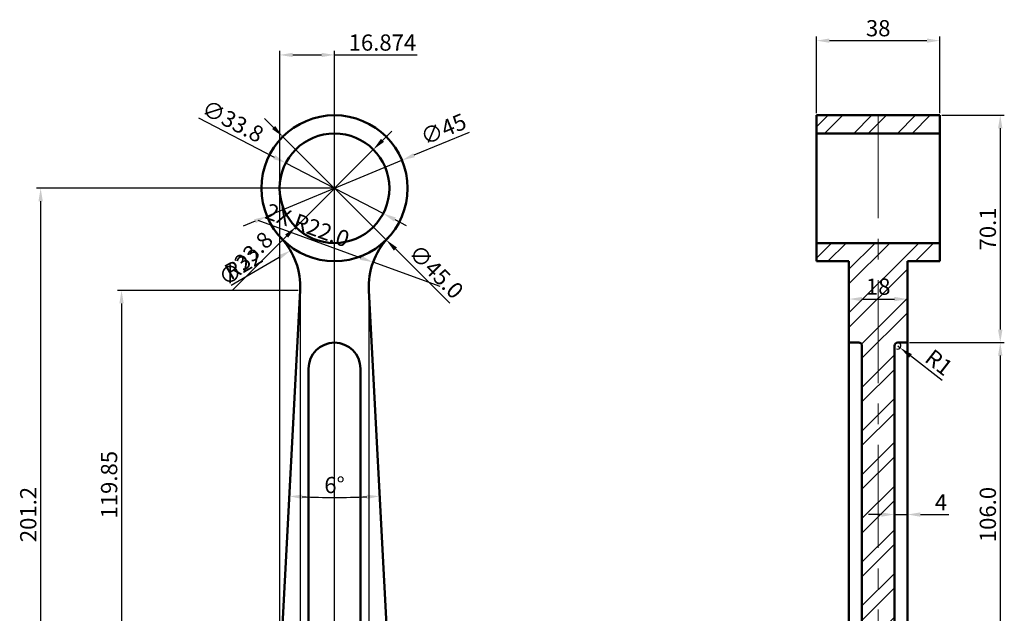
# Model space of a CAD drawing. Units: millimetres. Extents: x 3127 to 3430, y 1464 to 1830.
# Tile 2 of 2: x 3127 to 3430, y 1647 to 1830. Entities that reach past the tile are written whole.
import ezdxf

# ---------------------------------------------------------------- set-up
doc = ezdxf.new("R2010")
doc.units = ezdxf.units.MM
doc.linetypes.add('CENTER', pattern=[50.8, 31.75, -6.35, 6.35, -6.35])
for name, color, linetype, lineweight in [('M-CNTR', 1, 'CENTER', 18), ('M-DIMS', 2, 'Continuous', 25), ('M-HATC', 8, 'Continuous', 18), ('M-OUTL', 7, 'Continuous', 50)]:
    doc.layers.add(name, color=color, linetype=linetype, lineweight=lineweight)
doc.styles.get("Standard").update_dxf_attribs({"font": 'arial.ttf'})
doc.dimstyles.new('ISO-25', dxfattribs={"dimtxt": 5, "dimasz": 4, "dimexe": 1.25, "dimexo": 0.625, "dimtad": 1, "dimdsep": 46, "dimtxsty": 'Standard', "dimcen": 2.5, "dimadec": 0, "dimazin": 0, "dimtfac": 1, "dimtmove": 0, "dimatfit": 3, "dimfxl": 1, "dimarcsym": 0})

# ---------------------------------------------------------------- blocks, each defined once
blk = doc.blocks.new('*D3')
at = {"layer": 'Defpoints', "color": 0, "transparency": 16777216}
for p in [(3396.63, 1677.1), (3400.63, 1677.1), (3400.63, 1677.1)]:
    blk.add_point(p, dxfattribs=at)
at = {"layer": 'M-DIMS', "color": 0, "lineweight": -2, "transparency": 16777216}
for p, q in [((3396.63, 1677.72), (3396.63, 1678.35)), ((3400.63, 1677.72), (3400.63, 1678.35)), ((3392.63, 1677.1), (3388.63, 1677.1)), ((3396.63, 1677.1), (3400.63, 1677.1)), ((3404.63, 1677.1), (3413.34, 1677.1))]:
    blk.add_line(p, q, dxfattribs=at)
at = {"layer": 'M-DIMS', "color": 0, "transparency": 16777216}
for points in [[(3392.63, 1677.76), (3392.63, 1676.43), (3396.63, 1677.1)], [(3404.63, 1677.76), (3404.63, 1676.43), (3400.63, 1677.1)]]:
    blk.add_solid(points, dxfattribs=at)
at = {"layer": 'M-DIMS', "color": 0, "transparency": 16777216, "insert": (3410.98, 1680.22), "char_height": 5, "attachment_point": 5}
blk.add_mtext('4', dxfattribs=at)
blk = doc.blocks.new('*D12')
at = {"layer": 'Defpoints', "color": 0, "transparency": 16777216}
for p in [(3213.56, 1746.21), (3234.74, 1746.21), (3219.51, 1682.41), (3207.27, 1626.37), (3241.02, 1626.37)]:
    blk.add_point(p, dxfattribs=at)
at = {"layer": 'M-DIMS', "color": 0, "lineweight": -2, "transparency": 16777216}
blk.add_arc((3224.15, 1948.35), 265.98, 267.8617, 272.1383, dxfattribs=at)
at = {"layer": 'M-DIMS', "color": 0, "transparency": 16777216}
for points in [[(3214.19, 1681.89), (3214.25, 1683.22), (3210.23, 1682.73)], [(3234.04, 1683.22), (3234.1, 1681.89), (3238.07, 1682.73)]]:
    blk.add_solid(points, dxfattribs=at)
at = {"layer": 'M-DIMS', "color": 0, "transparency": 16777216, "insert": (3224.15, 1685.55), "char_height": 5, "attachment_point": 5}
blk.add_mtext('6°', dxfattribs=at)
blk = doc.blocks.new('*D13')
at = {"layer": 'Defpoints', "color": 0, "transparency": 16777216}
for p in [(3210.59, 1758.45), (3191.59, 1747.37)]:
    blk.add_point(p, dxfattribs=at)
at = {"layer": 'M-DIMS', "color": 0, "lineweight": -2, "transparency": 16777216}
blk.add_line((3192.32, 1747.8), (3207.13, 1756.43), dxfattribs=at)
at = {"layer": 'M-DIMS', "color": 0, "transparency": 16777216}
blk.add_solid([(3206.8, 1757.01), (3207.47, 1755.86), (3210.59, 1758.45)], dxfattribs=at)
at = {"layer": 'M-DIMS', "color": 0, "transparency": 16777216, "insert": (3196.42, 1753.82), "char_height": 5, "attachment_point": 5, "rotation": 30.2469}
blk.add_mtext('R22', dxfattribs=at)
blk = doc.blocks.new('*D14')
at = {"layer": 'Defpoints', "color": 0, "transparency": 16777216}
for p in [(3244.93, 1786.33), (3203.37, 1769.06)]:
    blk.add_point(p, dxfattribs=at)
at = {"layer": 'M-DIMS', "color": 0, "lineweight": -2, "transparency": 16777216}
for p, q in [((3265.64, 1794.93), (3248.62, 1787.86)), ((3203.37, 1769.06), (3244.93, 1786.33)), ((3199.68, 1767.53), (3195.98, 1766))]:
    blk.add_line(p, q, dxfattribs=at)
at = {"layer": 'M-DIMS', "color": 0, "transparency": 16777216}
for points in [[(3248.37, 1788.48), (3248.88, 1787.25), (3244.93, 1786.33)], [(3199.42, 1768.15), (3199.93, 1766.91), (3203.37, 1769.06)]]:
    blk.add_solid(points, dxfattribs=at)
at = {"layer": 'M-DIMS', "color": 0, "transparency": 16777216, "insert": (3257.95, 1795.33), "char_height": 5, "attachment_point": 5, "rotation": 22.5579}
blk.add_mtext('∅45', dxfattribs=at)
blk = doc.blocks.new('*D15')
at = {"layer": 'Defpoints', "color": 0, "transparency": 16777216}
for p in [(3209.14, 1785.47), (3239.16, 1769.92)]:
    blk.add_point(p, dxfattribs=at)
at = {"layer": 'M-DIMS', "color": 0, "lineweight": -2, "transparency": 16777216}
for p, q in [((3182.26, 1799.39), (3205.59, 1787.31)), ((3239.16, 1769.92), (3209.14, 1785.47)), ((3242.71, 1768.09), (3246.26, 1766.25))]:
    blk.add_line(p, q, dxfattribs=at)
at = {"layer": 'M-DIMS', "color": 0, "transparency": 16777216}
for points in [[(3205.9, 1787.9), (3205.28, 1786.71), (3209.14, 1785.47)], [(3243.01, 1768.68), (3242.4, 1767.49), (3239.16, 1769.92)]]:
    blk.add_solid(points, dxfattribs=at)
at = {"layer": 'M-DIMS', "color": 0, "transparency": 16777216, "insert": (3192.53, 1797.81), "char_height": 5, "attachment_point": 5, "rotation": 332.6249}
blk.add_mtext('∅33.8', dxfattribs=at)
blk = doc.blocks.new('*D16')
at = {"layer": 'Defpoints', "color": 0, "transparency": 16777216}
for p in [(3224.15, 1777.7), (3133.63, 1576.5), (3177.15, 1576.5)]:
    blk.add_point(p, dxfattribs=at)
at = {"layer": 'M-DIMS', "color": 0, "lineweight": -2, "transparency": 16777216}
for p, q in [((3223.52, 1777.7), (3132.38, 1777.7)), ((3133.63, 1773.7), (3133.63, 1580.5)), ((3176.52, 1576.5), (3132.38, 1576.5))]:
    blk.add_line(p, q, dxfattribs=at)
at = {"layer": 'M-DIMS', "color": 0, "transparency": 16777216}
for points in [[(3132.96, 1773.7), (3134.3, 1773.7), (3133.63, 1777.7)], [(3132.96, 1580.5), (3134.3, 1580.5), (3133.63, 1576.5)]]:
    blk.add_solid(points, dxfattribs=at)
at = {"layer": 'M-DIMS', "color": 0, "transparency": 16777216, "insert": (3130.45, 1677.1), "char_height": 5, "attachment_point": 5, "rotation": 90}
blk.add_mtext('201.2', dxfattribs=at)
blk = doc.blocks.new('*D17')
at = {"layer": 'Defpoints', "color": 0, "transparency": 16777216}
for p in [(3382.63, 1743.53), (3400.63, 1743.53), (3400.63, 1743.53)]:
    blk.add_point(p, dxfattribs=at)
at = {"layer": 'M-DIMS', "color": 0, "lineweight": -2, "transparency": 16777216}
for p, q in [((3382.63, 1744.15), (3382.63, 1744.78)), ((3400.63, 1744.15), (3400.63, 1744.78)), ((3386.63, 1743.53), (3396.63, 1743.53))]:
    blk.add_line(p, q, dxfattribs=at)
at = {"layer": 'M-DIMS', "color": 0, "transparency": 16777216}
for points in [[(3386.63, 1744.2), (3386.63, 1742.86), (3382.63, 1743.53)], [(3396.63, 1744.2), (3396.63, 1742.86), (3400.63, 1743.53)]]:
    blk.add_solid(points, dxfattribs=at)
at = {"layer": 'M-DIMS', "color": 0, "transparency": 16777216, "insert": (3391.63, 1746.71), "char_height": 5, "attachment_point": 5}
blk.add_mtext('18', dxfattribs=at)
blk = doc.blocks.new('*D18')
at = {"layer": 'Defpoints', "color": 0, "transparency": 16777216}
for p in [(3397.63, 1729.1), (3398.42, 1728.48)]:
    blk.add_point(p, dxfattribs=at)
at = {"layer": 'M-DIMS', "color": 0, "lineweight": -2, "transparency": 16777216}
for p, q in [((3397.63, 1729.1), (3398.42, 1728.48)), ((3411.32, 1718.44), (3401.58, 1726.03))]:
    blk.add_line(p, q, dxfattribs=at)
blk.add_arc((3397.63, 1729.1), 1, 250.5029, 54.1901, dxfattribs=at)
at = {"layer": 'M-DIMS', "color": 0, "transparency": 16777216}
blk.add_solid([(3401.99, 1726.55), (3401.17, 1725.5), (3398.42, 1728.48)], dxfattribs=at)
at = {"layer": 'M-DIMS', "color": 0, "transparency": 16777216, "insert": (3409.95, 1723.48), "char_height": 5, "attachment_point": 5, "rotation": 322.1226}
blk.add_mtext('R1', dxfattribs=at)
blk = doc.blocks.new('*D19')
at = {"layer": 'Defpoints', "color": 0, "transparency": 16777216}
for p in [(3410.63, 1823.21), (3372.63, 1800.2), (3410.63, 1800.2)]:
    blk.add_point(p, dxfattribs=at)
at = {"layer": 'M-DIMS', "color": 0, "lineweight": -2, "transparency": 16777216}
for p, q in [((3372.63, 1800.82), (3372.63, 1824.46)), ((3376.63, 1823.21), (3406.63, 1823.21)), ((3410.63, 1800.82), (3410.63, 1824.46))]:
    blk.add_line(p, q, dxfattribs=at)
at = {"layer": 'M-DIMS', "color": 0, "transparency": 16777216}
for points in [[(3376.63, 1823.88), (3376.63, 1822.54), (3372.63, 1823.21)], [(3406.63, 1823.88), (3406.63, 1822.54), (3410.63, 1823.21)]]:
    blk.add_solid(points, dxfattribs=at)
at = {"layer": 'M-DIMS', "color": 0, "transparency": 16777216, "insert": (3391.63, 1826.39), "char_height": 5, "attachment_point": 5}
blk.add_mtext('38', dxfattribs=at)
blk = doc.blocks.new('*D22')
at = {"layer": 'Defpoints', "color": 0, "transparency": 16777216}
for p in [(3410.63, 1800.2), (3400.63, 1730.1), (3429.23, 1730.1)]:
    blk.add_point(p, dxfattribs=at)
at = {"layer": 'M-DIMS', "color": 0, "lineweight": -2, "transparency": 16777216}
for p, q in [((3411.25, 1800.2), (3430.48, 1800.2)), ((3429.23, 1796.2), (3429.23, 1734.1)), ((3401.25, 1730.1), (3430.48, 1730.1))]:
    blk.add_line(p, q, dxfattribs=at)
at = {"layer": 'M-DIMS', "color": 0, "transparency": 16777216}
for points in [[(3428.56, 1796.2), (3429.9, 1796.2), (3429.23, 1800.2)], [(3428.56, 1734.1), (3429.9, 1734.1), (3429.23, 1730.1)]]:
    blk.add_solid(points, dxfattribs=at)
at = {"layer": 'M-DIMS', "color": 0, "transparency": 16777216, "insert": (3426.05, 1765.15), "char_height": 5, "attachment_point": 5, "rotation": 90}
blk.add_mtext('70.1', dxfattribs=at)
blk = doc.blocks.new('*D23')
at = {"layer": 'Defpoints', "color": 0, "transparency": 16777216}
for p in [(3400.63, 1730.1), (3400.63, 1624.1), (3429.23, 1624.1)]:
    blk.add_point(p, dxfattribs=at)
at = {"layer": 'M-DIMS', "color": 0, "lineweight": -2, "transparency": 16777216}
for p, q in [((3401.25, 1730.1), (3430.48, 1730.1)), ((3429.23, 1726.1), (3429.23, 1628.1)), ((3401.25, 1624.1), (3430.48, 1624.1))]:
    blk.add_line(p, q, dxfattribs=at)
at = {"layer": 'M-DIMS', "color": 0, "transparency": 16777216}
for points in [[(3428.56, 1726.1), (3429.9, 1726.1), (3429.23, 1730.1)], [(3428.56, 1628.1), (3429.9, 1628.1), (3429.23, 1624.1)]]:
    blk.add_solid(points, dxfattribs=at)
at = {"layer": 'M-DIMS', "color": 0, "transparency": 16777216, "insert": (3426.05, 1677.1), "char_height": 5, "attachment_point": 5, "rotation": 90}
blk.add_mtext('106.0', dxfattribs=at)
blk = doc.blocks.new('*D24')
at = {"layer": 'Defpoints', "color": 0, "transparency": 16777216}
for p in [(3213.56, 1746.21), (3234.74, 1746.21), (3234.74, 1469.62)]:
    blk.add_point(p, dxfattribs=at)
at = {"layer": 'M-DIMS', "color": 0, "lineweight": -2, "transparency": 16777216}
for p, q in [((3213.56, 1745.59), (3213.56, 1468.37)), ((3234.74, 1745.59), (3234.74, 1468.37)), ((3217.56, 1469.62), (3230.74, 1469.62)), ((3234.74, 1469.62), (3260.83, 1469.62))]:
    blk.add_line(p, q, dxfattribs=at)
at = {"layer": 'M-DIMS', "color": 0, "transparency": 16777216}
for points in [[(3217.56, 1470.29), (3217.56, 1468.96), (3213.56, 1469.62)], [(3230.74, 1470.29), (3230.74, 1468.96), (3234.74, 1469.62)]]:
    blk.add_solid(points, dxfattribs=at)
at = {"layer": 'M-DIMS', "color": 0, "transparency": 16777216, "insert": (3249.79, 1472.8), "char_height": 5, "attachment_point": 5}
blk.add_mtext('21.187', dxfattribs=at)
blk = doc.blocks.new('*D25')
at = {"layer": 'Defpoints', "color": 0, "transparency": 16777216}
for p in [(3224.15, 1818.8), (3207.27, 1626.37), (3224.15, 1603.5)]:
    blk.add_point(p, dxfattribs=at)
at = {"layer": 'M-DIMS', "color": 0, "lineweight": -2, "transparency": 16777216}
for p, q in [((3207.27, 1626.99), (3207.27, 1820.05)), ((3224.15, 1604.12), (3224.15, 1820.05)), ((3211.27, 1818.8), (3220.15, 1818.8)), ((3224.15, 1818.8), (3249.66, 1818.8))]:
    blk.add_line(p, q, dxfattribs=at)
at = {"layer": 'M-DIMS', "color": 0, "transparency": 16777216}
for points in [[(3211.27, 1819.46), (3211.27, 1818.13), (3207.27, 1818.8)], [(3220.15, 1819.46), (3220.15, 1818.13), (3224.15, 1818.8)]]:
    blk.add_solid(points, dxfattribs=at)
at = {"layer": 'M-DIMS', "color": 0, "transparency": 16777216, "insert": (3238.91, 1821.97), "char_height": 5, "attachment_point": 5}
blk.add_mtext('16.874', dxfattribs=at)
blk = doc.blocks.new('*D26')
at = {"layer": 'Defpoints', "color": 0, "transparency": 16777216}
for p in [(3213.56, 1746.21), (3158.55, 1626.37), (3207.27, 1626.37)]:
    blk.add_point(p, dxfattribs=at)
at = {"layer": 'M-DIMS', "color": 0, "lineweight": -2, "transparency": 16777216}
for p, q in [((3212.93, 1746.21), (3157.3, 1746.21)), ((3158.55, 1742.21), (3158.55, 1630.37)), ((3206.65, 1626.37), (3157.3, 1626.37))]:
    blk.add_line(p, q, dxfattribs=at)
at = {"layer": 'M-DIMS', "color": 0, "transparency": 16777216}
for points in [[(3157.88, 1742.21), (3159.22, 1742.21), (3158.55, 1746.21)], [(3157.88, 1630.37), (3159.22, 1630.37), (3158.55, 1626.37)]]:
    blk.add_solid(points, dxfattribs=at)
at = {"layer": 'M-DIMS', "color": 0, "transparency": 16777216, "insert": (3155.37, 1686.29), "char_height": 5, "attachment_point": 5, "rotation": 90}
blk.add_mtext('119.85', dxfattribs=at)
blk = doc.blocks.new('*D28')
at = {"layer": 'Defpoints', "color": 0, "transparency": 16777216}
for p in [(3208.23, 1793.6), (3240.07, 1761.79)]:
    blk.add_point(p, dxfattribs=at)
at = {"layer": 'M-DIMS', "color": 0, "lineweight": -2, "transparency": 16777216}
for p, q in [((3205.4, 1796.42), (3202.57, 1799.25)), ((3208.23, 1793.6), (3240.07, 1761.79)), ((3259.64, 1742.24), (3242.9, 1758.97))]:
    blk.add_line(p, q, dxfattribs=at)
at = {"layer": 'M-DIMS', "color": 0, "transparency": 16777216}
for points in [[(3205.87, 1796.9), (3204.93, 1795.95), (3208.23, 1793.6)], [(3243.37, 1759.44), (3242.43, 1758.49), (3240.07, 1761.79)]]:
    blk.add_solid(points, dxfattribs=at)
at = {"layer": 'M-DIMS', "color": 0, "transparency": 16777216, "insert": (3255.03, 1751.54), "char_height": 5, "attachment_point": 5, "rotation": 315.0282}
blk.add_mtext('∅45.0', dxfattribs=at)
blk = doc.blocks.new('*D29')
at = {"layer": 'Defpoints', "color": 0, "transparency": 16777216}
for p in [(3236.1, 1789.64), (3212.2, 1765.75)]:
    blk.add_point(p, dxfattribs=at)
at = {"layer": 'M-DIMS', "color": 0, "lineweight": -2, "transparency": 16777216}
for p, q in [((3238.93, 1792.47), (3241.76, 1795.3)), ((3236.1, 1789.64), (3212.2, 1765.75)), ((3192.62, 1746.17), (3209.37, 1762.92))]:
    blk.add_line(p, q, dxfattribs=at)
at = {"layer": 'M-DIMS', "color": 0, "transparency": 16777216}
for points in [[(3238.46, 1792.94), (3239.4, 1792), (3236.1, 1789.64)], [(3208.9, 1763.39), (3209.84, 1762.45), (3212.2, 1765.75)]]:
    blk.add_solid(points, dxfattribs=at)
at = {"layer": 'M-DIMS', "color": 0, "transparency": 16777216, "insert": (3197.23, 1755.48), "char_height": 5, "attachment_point": 5, "rotation": 44.993}
blk.add_mtext('∅33.8', dxfattribs=at)
blk = doc.blocks.new('*D30')
at = {"layer": 'Defpoints', "color": 0, "transparency": 16777216}
for p in [(3236.04, 1754.88), (3256.71, 1747.37)]:
    blk.add_point(p, dxfattribs=at)
at = {"layer": 'M-DIMS', "color": 0, "lineweight": -2, "transparency": 16777216}
for p, q in [((3200.48, 1767.81), (3232.28, 1756.25)), ((3256.71, 1747.37), (3236.04, 1754.88))]:
    blk.add_line(p, q, dxfattribs=at)
at = {"layer": 'M-DIMS', "color": 0, "transparency": 16777216}
blk.add_solid([(3232.51, 1756.88), (3232.05, 1755.62), (3236.04, 1754.88)], dxfattribs=at)
at = {"layer": 'M-DIMS', "color": 0, "transparency": 16777216, "insert": (3215.58, 1765.7), "char_height": 5, "attachment_point": 5, "rotation": 340.0179}
blk.add_mtext('2X R22.0', dxfattribs=at)

msp = doc.modelspace()

# ---------------------------------------------------------------- hatches: boundary and pattern name
at = {"layer": 'M-HATC'}
h = msp.add_hatch(dxfattribs=at)
h.set_pattern_fill('ANSI32', color=256)
h.paths.add_polyline_path([(3391.6295, 1800.1957), (3372.6295, 1800.1957), (3372.6295, 1794.5957), (3391.6295, 1794.5957)])
h.paths.add_polyline_path([(3410.6295, 1800.1957), (3391.6295, 1800.1957), (3391.6295, 1794.5957), (3410.6295, 1794.5957)])
h.paths.add_polyline_path([(3400.6295, 1755.1957), (3410.6295, 1755.1957), (3410.6295, 1760.7957), (3391.6295, 1760.7957), (3391.6295, 1603.4957), (3410.6295, 1603.4957), (3410.6295, 1613.4957), (3403.6295, 1613.4957, -0.41421356), (3400.6295, 1616.4957), (3400.6295, 1624.0957), (3397.6295, 1624.0957, -0.41421356), (3396.6295, 1625.0957), (3396.6295, 1729.0957, -0.41421356), (3397.6295, 1730.0957), (3400.6295, 1730.0957)])
h.paths.add_polyline_path([(3391.6295, 1760.7957), (3372.6295, 1760.7957), (3372.6295, 1755.1957), (3382.6295, 1755.1957), (3382.6295, 1730.0957), (3385.6295, 1730.0957, -0.41421356), (3386.6295, 1729.0957), (3386.6295, 1625.0957, -0.41421356), (3385.6295, 1624.0957), (3382.6295, 1624.0957), (3382.6295, 1616.4957, -0.41421356), (3379.6295, 1613.4957), (3372.6295, 1613.4957), (3372.6295, 1603.4957), (3391.6295, 1603.4957)])
h.paths.add_polyline_path([(3262.1486, 1526.2219), (3251.1486, 1526.2219), (3251.1486, 1507.2219), (3257.6486, 1507.2219, -1), (3266.6486, 1507.2219), (3271.1486, 1507.2219, 0.41421356), (3262.1486, 1516.2219)])
h.paths.add_polyline_path([(3271.1486, 1507.2219), (3266.6486, 1507.2219, -1), (3257.6486, 1507.2219), (3251.1486, 1507.2219), (3251.1486, 1488.2219), (3262.1486, 1488.2219), (3262.1486, 1498.2219, 0.41421356)])
h.paths.add_polyline_path([(3197.1486, 1526.2219), (3186.1486, 1526.2219), (3186.1486, 1516.2219, 0.41421356), (3177.1486, 1507.2219), (3181.6486, 1507.2219, -1), (3190.6486, 1507.2219), (3197.1486, 1507.2219)])
h.paths.add_polyline_path([(3197.1486, 1507.2219), (3190.6486, 1507.2219, -1), (3181.6486, 1507.2219), (3177.1486, 1507.2219, 0.41421356), (3186.1486, 1498.2219), (3186.1486, 1488.2219), (3197.1486, 1488.2219)])

# ---------------------------------------------------------------- linework, layer by layer
at = {"layer": 'M-CNTR'}
for p, q in [((3391.6295, 1800.1957), (3391.6295, 1576.4957)), ((3224.1486, 1777.6957), (3224.1486, 1624.0957))]:
    msp.add_line(p, q, dxfattribs=at)
at = {"layer": 'M-OUTL'}
for p, q in [((3372.6295, 1800.1957), (3410.6295, 1800.1957)), ((3372.6295, 1800.1957), (3372.6295, 1755.1957)), ((3410.6295, 1800.1957), (3410.6295, 1755.1957)), ((3372.6295, 1794.5957), (3410.6295, 1794.5957)), ((3239.0026, 1760.7957), (3239.2865, 1760.7957)), ((3372.6295, 1760.7957), (3410.6295, 1760.7957)), ((3372.6295, 1755.1957), (3382.6295, 1755.1957)), ((3382.6295, 1755.1957), (3382.6295, 1616.4957)), ((3400.6295, 1755.1957), (3400.6295, 1616.4957)), ((3400.6295, 1755.1957), (3410.6295, 1755.1957)), ((3213.5551, 1746.2148), (3207.2742, 1626.369)), ((3234.7422, 1746.2148), (3241.023, 1626.369)), ((3382.6295, 1730.0957), (3385.6295, 1730.0957)), ((3386.6295, 1729.0957), (3386.6295, 1625.0957)), ((3396.6295, 1729.0957), (3396.6295, 1625.0957)), ((3397.6295, 1730.0957), (3400.6295, 1730.0957)), ((3216.1486, 1722.0957), (3216.1486, 1632.0957)), ((3232.1486, 1722.0957), (3232.1486, 1632.0957))]:
    msp.add_line(p, q, dxfattribs=at)
for radius in [22.5, 16.9]:
    msp.add_circle((3224.1486, 1777.6957), radius, dxfattribs=at)
for centre, radius, start, end in [((3191.5853, 1747.3662), 22, 357, 42.965744), ((3256.712, 1747.3662), 22, 137.034256, 183), ((3224.1486, 1722.0957), 8, 0, 180), ((3385.6295, 1729.0957), 1, 0, 90), ((3397.6295, 1729.0957), 1, 90, 180)]:
    msp.add_arc(centre, radius, start, end, dxfattribs=at)

# ---------------------------------------------------------------- dimensions: what is measured, and where the dimension line sits
at = {"layer": 'M-DIMS'}
for base, p1, p2, override, picture, middle in [((3410.6295, 1823.2101), (3372.6295, 1800.1957), (3410.6295, 1800.1957), {"dimclrd": 0, "dimclre": 0, "dimclrt": 0}, '*D19', (3391.6295, 1826.3896)), ((3224.1486, 1818.7957), (3207.2742, 1626.369), (3224.1486, 1603.4957), {"dimdec": 3, "dimlfac": 1, "dimrnd": 0, "dimzin": 0, "dimdsep": 46, "dimlunit": 2}, '*D25', (3238.9067, 1821.9736)), ((3400.6295, 1743.5294), (3382.6295, 1743.5294), (3400.6295, 1743.5294), {"dimclrd": 0, "dimclre": 0, "dimclrt": 0}, '*D17', (3391.6295, 1746.7073)), ((3234.7422, 1469.6219), (3213.5551, 1746.2148), (3234.7422, 1746.2148), {"dimdec": 3, "dimlfac": 1, "dimrnd": 0, "dimzin": 0, "dimdsep": 46, "dimlunit": 2}, '*D24', (3249.7884, 1472.7997)), ((3400.6295, 1677.0957), (3396.6295, 1677.0957), (3400.6295, 1677.0957), {"dimclrd": 0, "dimclre": 0, "dimclrt": 0}, '*D3', (3410.9837, 1680.2207))]:
    dim = msp.add_linear_dim(base=base, p1=p1, p2=p2, dimstyle='ISO-25', override=override, dxfattribs=at)
    dim.commit()
    dim.dimension.update_dxf_attribs({"geometry": picture, "text_midpoint": middle})
for p1, p2, override, picture, middle in [((3239.1561, 1769.9249), (3209.1412, 1785.4665), {"dimclrd": 0, "dimclre": 0, "dimclrt": 0}, '*D15', (3190.9999, 1794.8601)), ((3203.3701, 1769.0643), (3244.9272, 1786.3271), {"dimclrd": 0, "dimclre": 0, "dimclrt": 0}, '*D14', (3259.2215, 1792.2649)), ((3208.2309, 1793.5978), (3240.0664, 1761.7936), {"dimdec": 1, "dimlfac": 1, "dimrnd": 0, "dimzin": 0, "dimdsep": 46, "dimlunit": 2}, '*D28', (3252.6805, 1749.1919)), ((3236.1002, 1789.6443), (3212.1971, 1765.7471), {"dimdec": 1, "dimlfac": 1, "dimrnd": 0, "dimzin": 0, "dimdsep": 46, "dimlunit": 2}, '*D29', (3199.5779, 1753.131))]:
    dim = msp.add_diameter_dim_2p(p1=p1, p2=p2, dimstyle='ISO-25', override=override, dxfattribs=at)
    dim.commit()
    dim.dimension.update_dxf_attribs({"geometry": picture, "text_midpoint": middle, "dimtype": 163})
for base, p1, p2, override, picture, middle in [((3429.2295, 1730.0957), (3410.6295, 1800.1957), (3400.6295, 1730.0957), {"dimdec": 1, "dimlfac": 1, "dimrnd": 0, "dimzin": 0, "dimdsep": 46, "dimlunit": 2}, '*D22', (3426.0516, 1765.1457)), ((3133.6315, 1576.4957), (3224.1486, 1777.6957), (3177.1486, 1576.4957), {"dimclrd": 0, "dimclre": 0, "dimclrt": 0}, '*D16', (3130.4537, 1677.0957)), ((3158.5486, 1626.369), (3213.5551, 1746.2148), (3207.2742, 1626.369), {"dimdec": 2, "dimlfac": 1, "dimrnd": 0, "dimzin": 0, "dimdsep": 46, "dimlunit": 2}, '*D26', (3155.3708, 1686.2919)), ((3429.2295, 1624.0957), (3400.6295, 1730.0957), (3400.6295, 1624.0957), {"dimdec": 1, "dimlfac": 1, "dimrnd": 0, "dimzin": 0, "dimdsep": 46, "dimlunit": 2}, '*D23', (3426.0516, 1677.0957))]:
    dim = msp.add_linear_dim(base=base, p1=p1, p2=p2, angle=90, dimstyle='ISO-25', override=override, dxfattribs=at)
    dim.commit()
    dim.dimension.update_dxf_attribs({"geometry": picture, "text_midpoint": middle})
dim = msp.add_radius_dim(center=(3256.712, 1747.3662), mpoint=(3236.0364, 1754.8842), text='2X <>', dimstyle='ISO-25', override={"dimdec": 1, "dimlfac": 1, "dimrnd": 0, "dimzin": 0, "dimdsep": 46, "dimlunit": 2}, dxfattribs=at)
dim.commit()
dim.dimension.update_dxf_attribs({"geometry": '*D30', "text_midpoint": (3215.5847, 1765.7022)})
dim = msp.add_radius_dim(center=(3191.5853, 1747.3662), mpoint=(3210.5902, 1758.4482), dimstyle='ISO-25', override={"dimclrd": 0, "dimclre": 0, "dimclrt": 0}, dxfattribs=at)
dim.commit()
dim.dimension.update_dxf_attribs({"geometry": '*D13', "text_midpoint": (3198.001, 1751.1073), "dimtype": 164})
dim = msp.add_angular_dim_2l(base=(3219.5066, 1682.4079), line1=((3234.7422, 1746.2148), (3241.023, 1626.369)), line2=((3213.5551, 1746.2148), (3207.2742, 1626.369)), dimstyle='ISO-25', override={"dimclrd": 0, "dimclre": 0, "dimclrt": 0}, dxfattribs=at)
dim.commit()
dim.dimension.update_dxf_attribs({"geometry": '*D12', "text_midpoint": (3224.1486, 1685.5453)})
dim = msp.add_radius_dim(center=(3397.6295, 1729.0957), mpoint=(3398.4188, 1728.4817), dimstyle='ISO-25', override={"dimclrd": 0, "dimclre": 0, "dimclrt": 0}, dxfattribs=at)
dim.commit()
dim.dimension.update_dxf_attribs({"geometry": '*D18', "text_midpoint": (3409.9528, 1723.4821)})

doc.saveas('drawing.dxf')
